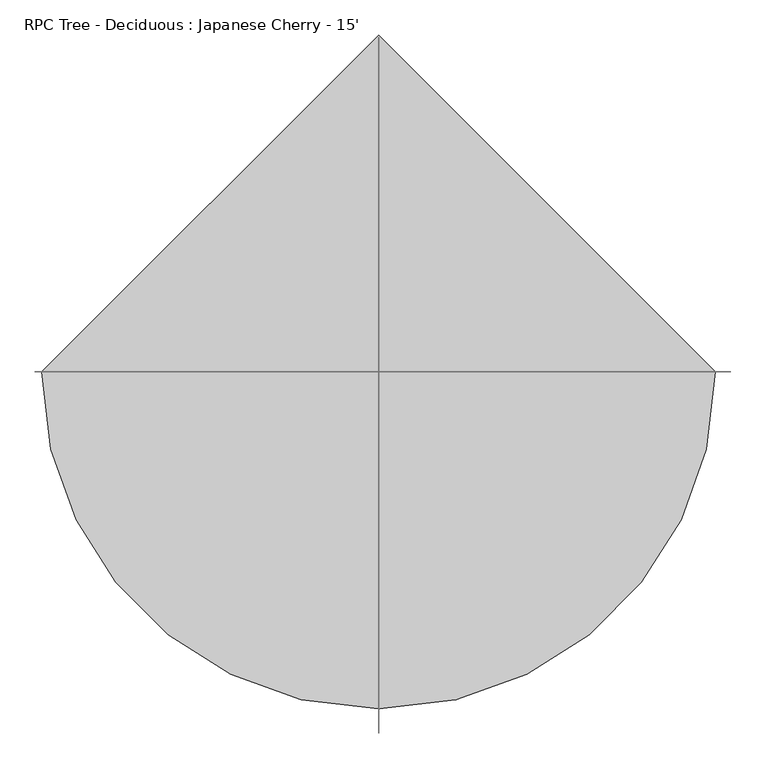
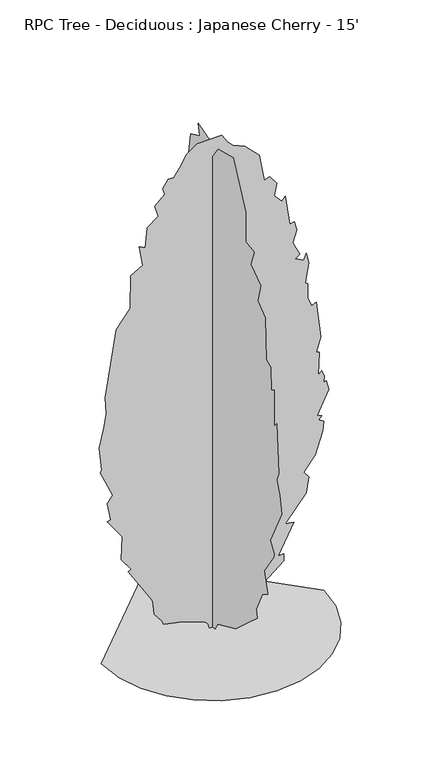
"""IFC4 building model written with IfcOpenShell, lengths in millimetres: geographic element geometry, RPC Tree - Deciduous : Japanese Cherry - 15'."""

from ifc_helpers import new_model, si_unit, origin, place, context, project, spatial, triangles, source, transform, mapped, element, save


def rpc_tree_deciduous_japanese_cherry_15_056c1364(model_context):
    return source(origin(), model_context, "Body", "Tessellation", [
        triangles([(-18.9184083, 8e-07, 1.7e-06), (-23.4048623, -4e-07, 23.0653231), (-35.5101849, -8e-07, 39.0747225), (-159.1266788, 1.9e-06, 84.5688842), (-259.5506544, 5e-06, 105.8783847), (-269.176048, 4e-06, 129.9415507), (-307.9581648, 2.8e-06, 179.5870942), (-317.3030522, -1.3e-06, 255.0704046), (-331.7421055, -2.4e-06, 283.9462765), (-447.244285, -8.3e-06, 466.8255389), (-432.3003207, -9.5e-06, 475.8063134), (-483.4056315, -1.15e-05, 547.4497602), (-478.2261875, -1.93e-05, 674.5223454), (-557.9360023, -2.24e-05, 784.4630184), (-538.6845612, -2.35e-05, 789.2734079), (-557.1881556, -2.85e-05, 886.5267014), (-529.0572055, -3.2e-05, 924.0270287), (-596.4356509, -3.79e-05, 1073.2216284), (-586.8115291, -3.89e-05, 1082.8457502), (-601.2493106, -4.6e-05, 1212.7856386), (-575.1300473, -5.39e-05, 1326.1552448), (-562.7464282, -5.83e-05, 1390.8558014), (-567.5600879, -6.35e-05, 1482.2961502), (-509.8090344, -8.76e-05, 1843.2435951), (-437.6201632, -9.65e-05, 1939.4976036), (-433.7176397, -0.0001074, 2119.1484112), (-370.2417541, -0.0001123, 2156.0673786), (-389.4931952, -0.0001181, 2266.7558258), (-356.6367342, -0.0001184, 2247.9061043), (-346.179887, -0.0001254, 2358.1961746), (-288.4265263, -0.0001305, 2401.5095192), (-307.6773316, -0.0001334, 2464.074305), (-254.7379576, -0.0001386, 2512.2013092), (-264.3633512, -0.0001402, 2545.8905319), (-235.4874975, -0.000144, 2589.2035858), (-206.6116256, -0.0001453, 2589.2035858), (-173.4808535, -0.0001493, 2632.2198555), (-140.2658206, -0.0001545, 2694.6605209), (-80.6725468, -0.0001595, 2735.0150345), (47.4656756, -0.0001652, 2737.0300278), (77.3346509, -0.0001637, 2690.2680565), (106.2105138, -0.0001633, 2661.3924934), (170.4097655, -0.0001645, 2634.2022926), (245.777131, -0.0001631, 2555.5146538), (274.6530029, -0.0001554, 2406.3231789), (303.5288748, -0.0001573, 2415.9473007), (338.7470922, -0.0001558, 2365.5636028), (327.5913777, -0.0001514, 2300.4450485), (366.0942601, -0.0001505, 2257.1318493), (385.3424675, -0.0001525, 2276.3832905), (409.4075684, -0.0001438, 2112.7508366), (433.4694354, -0.0001452, 2117.5644962), (446.5551919, -0.0001429, 2069.8881912), (425.0471297, -0.0001381, 2004.4658764), (462.3449621, -0.000135, 1925.0598221), (437.127061, -0.0001329, 1909.9395241), (481.5964396, -0.0001335, 1886.5569397), (496.0341848, -0.0001361, 1920.2461624), (510.4719664, -0.0001333, 1862.4950363), (491.2237953, -0.0001262, 1756.6170513), (505.1194588, -0.0001261, 1745.1837376), (503.1894167, -0.0001214, 1667.0088581), (524.9097479, -0.0001193, 1617.0496983), (548.9748487, -0.000121, 1626.6738201), (573.0367158, -0.00011, 1424.5450241), (548.9748487, -0.0001043, 1347.5424568), (563.9612523, -0.0001047, 1342.4511978), (558.5989343, -9.7e-05, 1217.599371), (577.8504118, -9.87e-05, 1232.0371525), (592.288157, -9.73e-05, 1198.3479298), (587.4744973, -9.51e-05, 1164.6619772), (601.9122425, -9.6e-05, 1169.4723667), (616.350024, -9.35e-05, 1116.534973), (553.7852746, -8.33e-05, 991.4054741), (577.8504118, -8.38e-05, 981.7813522), (563.4126303, -8.2e-05, 962.529911), (587.4744973, -8.22e-05, 948.0921295), (582.412597, -7.89e-05, 896.2226212), (544.1611891, -7e-05, 774.8356264), (481.5964396, -6.26e-05, 697.8331318), (510.4719664, -6.19e-05, 664.1439091), (494.6887001, -5.62e-05, 580.0710975), (385.3424675, -4.32e-05, 442.7637082), (428.6590459, -4.48e-05, 437.9500122), (346.8428189, -3.18e-05, 279.1335797), (375.718382, -3.31e-05, 279.1335797), (375.718382, -3.08e-05, 240.6323143), (163.9615944, -1.12e-05, 67.3771283), (163.9615944, -1.26e-05, 91.4402943), (19.5827868, -9e-07, 0.0), (1.4e-06, 17.7289335, 0.0001671), (3.3e-06, 44.3328681, 18.3810013), (6.6e-06, 99.5438604, 38.501588), (9.2e-06, 229.4854111, 86.6279245), (1.49e-05, 296.8625484, 149.192347), (1.39e-05, 267.9866765, 154.0050437), (2.49e-05, 370.9863307, 302.4727256), (2.67e-05, 340.1774918, 375.3852628), (3.08e-05, 426.8041082, 500.5147616), (3.29e-05, 417.1800227, 558.2658514), (3.9e-05, 479.741502, 635.268346), (4.39e-05, 500.7760102, 727.3683203), (4.25e-05, 489.3688577, 822.9626307), (5.09e-05, 566.3713886, 938.4648102), (5.61e-05, 571.1817781, 1053.9701872), (5.9e-05, 543.3839473, 1148.493342), (6.23e-05, 585.6195597, 1299.4155979), (6.3e-05, 547.1199111, 1352.352919), (6.76e-05, 498.9929432, 1506.3580536), (6.85e-05, 532.6821659, 1612.2360386), (7.36e-05, 494.1792472, 1766.2410278), (7.55e-05, 446.0555494, 1857.6813766), (7.77e-05, 421.9904122, 2050.1893936), (7.58e-05, 393.1148855, 2035.7516121), (8.33e-05, 393.1148855, 2209.004845), (8.14e-05, 335.3637958, 2223.4426266), (7.94e-05, 304.8109732, 2326.2475433), (8.24e-05, 287.2371367, 2411.1368385), (8.24e-05, 229.4854111, 2468.8879646), (8.87e-05, 200.6095573, 2642.1442497), (8.16e-05, 118.7943296, 2680.6439346), (8.49e-05, 131.2197612, 2742.5948044), (7.82e-05, 14.5912583, 2705.4145157), (7.94e-05, 8.1035365, 2622.8928085), (7.53e-05, -49.6481596, 2704.7090355), (7.09e-05, -189.2147768, 2743.2087204), (6.07e-05, -304.7185733, 2507.3876495), (5.36e-05, -304.7185733, 2343.7583931), (4.96e-05, -380.8357658, 2330.2089294), (4.73e-05, -348.0315545, 2242.6940678), (4.56e-05, -440.7977308, 2179.3682819), (4.23e-05, -415.4099999, 2079.0648113), (3.71e-05, -482.7851389, 2026.1241474), (3.17e-05, -492.4124946, 1795.1165909), (2.93e-05, -531.7056993, 1778.3536606), (2.35e-05, -535.7258028, 1650.738921), (2.31e-05, -564.6013659, 1669.9871647), (1.94e-05, -564.6013659, 1467.8583687), (1.45e-05, -588.6631966, 1496.7339317), (7e-06, -607.9146741, 1227.2266903), (5.9e-06, -587.0172941, 1181.3857384), (1.5e-06, -617.5420298, 1111.7213133), (1.9e-06, -631.9798113, 1015.4673048), (-2.8e-06, -530.9121431, 808.5248491), (-6.8e-06, -564.6013659, 750.7737957), (-2.4e-06, -561.7536472, 730.3858686), (-4.1e-06, -473.1610534, 601.5824298), (-1.04e-05, -506.8502761, 490.8906761), (-9.6e-06, -453.9096122, 457.2014534), (-7.2e-06, -400.9722184, 341.6993102), (-9.5e-06, -410.5963039, 298.3843669), (-9.1e-06, -314.3436399, 211.7567694), (-8.6e-06, -213.277952, 120.3164841), (-4.7e-06, -44.8348088, 43.3139623), (-3e-07, -20.7722627, 0.0001648), (-589.06815, 0.0, 0.0001918), (-573.493919, -134.9753459, 0.0001831), (-529.1421204, -258.9288719, 0.0001738), (-459.5625738, -368.3084418, 0.0001642), (-368.3084418, -459.5625738, 0.0001548), (-258.9288719, -529.1421204, 0.0001459), (-134.9753459, -573.493919, 0.0001378), (2.65e-05, -589.06815, 0.000131), (134.9753459, -573.493919, 0.000126), (258.9288719, -529.1421204, 0.0001232), (368.3084418, -459.5625738, 0.0001226), (459.5625738, -368.3084418, 0.000124), (529.1421204, -258.9285449, 0.0001275), (573.493919, -134.9753459, 0.000133), (589.06815, 5.15e-05, 0.0001403), (-7.69e-05, 589.06815, 0.0002012)], [[57, 58, 59], [27, 28, 29], [87, 88, 89], [49, 50, 51], [13, 14, 15], [83, 84, 85], [74, 75, 76], [63, 64, 65], [68, 69, 70], [71, 72, 73], [9, 10, 11], [85, 86, 87], [85, 87, 89], [51, 52, 53], [54, 55, 56], [90, 1, 2], [66, 67, 68], [45, 46, 47], [17, 18, 19], [68, 70, 71], [45, 47, 48], [31, 32, 33], [76, 77, 78], [89, 90, 2], [89, 2, 3], [57, 59, 60], [51, 53, 54], [25, 26, 27], [39, 40, 41], [56, 57, 60], [71, 73, 74], [34, 35, 36], [33, 34, 36], [4, 5, 6], [60, 61, 62], [80, 81, 82], [38, 39, 41], [37, 38, 41], [37, 41, 42], [29, 30, 31], [15, 16, 17], [36, 37, 42], [33, 36, 42], [31, 33, 42], [31, 42, 43], [31, 43, 44], [31, 44, 45], [29, 31, 45], [29, 45, 48], [27, 29, 48], [25, 27, 48], [25, 48, 49], [25, 49, 51], [25, 51, 54], [25, 54, 56], [25, 56, 60], [25, 60, 62], [24, 25, 62], [23, 24, 62], [22, 23, 62], [22, 62, 63], [22, 63, 65], [22, 65, 66], [22, 66, 68], [21, 22, 68], [20, 21, 68], [19, 20, 68], [17, 19, 68], [17, 68, 71], [17, 71, 74], [15, 17, 74], [13, 15, 74], [13, 74, 76], [13, 76, 78], [13, 78, 79], [13, 79, 80], [12, 13, 80], [11, 12, 80], [9, 11, 80], [9, 80, 82], [9, 82, 83], [9, 83, 85], [9, 85, 89], [9, 89, 3], [9, 3, 4], [8, 9, 4], [8, 4, 6], [7, 8, 6], [138, 139, 140], [94, 95, 96], [136, 137, 138], [121, 122, 123], [112, 113, 114], [128, 129, 130], [121, 123, 124], [125, 126, 127], [124, 125, 127], [114, 115, 116], [147, 148, 149], [130, 131, 132], [124, 127, 128], [134, 135, 136], [154, 155, 91], [154, 91, 92], [150, 151, 152], [96, 97, 98], [119, 120, 121], [119, 121, 124], [119, 124, 128], [118, 119, 128], [117, 118, 128], [116, 117, 128], [116, 128, 130], [114, 116, 130], [114, 130, 132], [112, 114, 132], [112, 132, 133], [112, 133, 134], [112, 134, 136], [111, 112, 136], [110, 111, 136], [109, 110, 136], [109, 136, 138], [109, 138, 140], [109, 140, 141], [108, 109, 141], [107, 108, 141], [106, 107, 141], [105, 106, 141], [104, 105, 141], [103, 104, 141], [103, 141, 142], [103, 142, 143], [103, 143, 144], [102, 103, 144], [101, 102, 144], [100, 101, 144], [100, 144, 145], [100, 145, 146], [100, 146, 147], [100, 147, 149], [100, 149, 150], [100, 150, 152], [100, 152, 153], [100, 153, 154], [99, 100, 154], [98, 99, 154], [96, 98, 154], [96, 154, 92], [96, 92, 93], [96, 93, 94], [170, 171, 156], [169, 170, 156], [169, 156, 157], [168, 169, 157], [168, 157, 158], [168, 158, 159], [167, 168, 159], [166, 167, 159], [166, 159, 160], [166, 160, 161], [166, 161, 162], [166, 162, 163], [166, 163, 164], [166, 164, 165]], closed=False),
    ])


if __name__ == "__main__":
    model = new_model("IFC4")
    model_context = context("Model", 3, world=origin())
    ifc_project = project(units=[si_unit("LENGTHUNIT", "METRE", prefix="MILLI")], contexts=[model_context])
    site = spatial("IfcSite", under=ifc_project)
    building = spatial("IfcBuilding", under=site)
    placement = place(None, origin())
    rpc_tree_deciduous_japanese_cherry_15_shape = rpc_tree_deciduous_japanese_cherry_15_056c1364(model_context)
    element("IfcGeographicElement", 1, ObjectType="RPC Tree - Deciduous : Japanese Cherry - 15'", at=placement, inside=building, context=model_context, shape_type="MappedRepresentation", body=[
        mapped(rpc_tree_deciduous_japanese_cherry_15_shape, transform((0.0, 0.0, 0.0), x_axis=(1.0, 0.0, 0.0), y_axis=(0.0, 1.0, 0.0), z_axis=(0.0, 0.0, 1.0))),
    ])
    save(model, "model.ifc")

# Revit data of these elements
# Type "RPC Tree - Deciduous : Japanese Cherry - 15'"
#   built-in parameter 1005195 = "RPC-16-FUM3-UUQ0-UBF0-N000-ST1L-LVER-AU"
#   Type Comments = "Japanese Cherry"
#   Assembly Code = "G2050500"
#   Height = 9' - 0"
#   Default Elevation = 0
